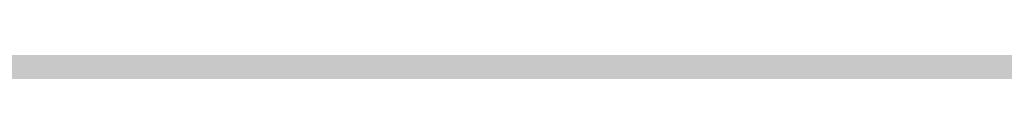
# Model space of a CAD drawing. Units: feet. Extents: x 3168 to 4724, y 827 to 1477.
# Tile 239 of 256: x 3382.8822 to 3383.8327, y 1099.0007 to 1099.0148. Entities that reach past the tile are written whole.
import ezdxf

# ---------------------------------------------------------------- set-up
doc = ezdxf.new("R2010")
doc.units = ezdxf.units.FT
doc.layers.add('A-ELEV', color=7, linetype='Continuous', lineweight=35)
doc.layers.add('A-ELEV-PATT', color=8, linetype='Continuous', lineweight=13)

msp = doc.modelspace()

# ---------------------------------------------------------------- hatches: boundary and pattern name
at = {"layer": 'A-ELEV-PATT'}
h = msp.add_hatch(color=256, dxfattribs=at)
h.dxf.hatch_style = 1
edge = h.paths.add_edge_path()
edge.add_ellipse((3552.90576, 979.22014), major_axis=(36.74492, 0), ratio=0.48484848, start_angle=0, end_angle=360)
edge = h.paths.add_edge_path()
edge.add_ellipse((3559.89164, 929.25228), major_axis=(36.74492, 0), ratio=0.48484848, start_angle=0, end_angle=360)
edge = h.paths.add_edge_path()
edge.add_line((3299.31681, 1198.60608), (3479.91671, 1198.60608))
edge.add_line((3479.91671, 1198.60608), (3479.91671, 1209.86857))
edge.add_spline(control_points=[(3479.91671, 1209.86857), (3464.30116, 1209.86857), (3448.6856, 1209.86857), (3410.94914, 1209.86857), (3388.82823, 1209.86857), (3355.64688, 1209.86857), (3344.58642, 1209.86857), (3327.99574, 1209.86857), (3322.46552, 1209.86857), (3314.17018, 1209.86857), (3311.40507, 1209.86857), (3307.2574, 1209.86857), (3305.87484, 1209.86857), (3303.801, 1209.86857), (3303.10973, 1209.86857), (3302.07281, 1209.86857), (3301.72717, 1209.86857), (3301.20871, 1209.86857), (3301.03589, 1209.86857), (3300.77666, 1209.86857), (3300.69025, 1209.86857), (3300.56064, 1209.86857), (3300.51743, 1209.86857), (3300.45263, 1209.86857), (3300.43102, 1209.86857), (3300.39862, 1209.86857), (3300.38782, 1209.86857), (3300.36622, 1209.86857), (3300.34568, 1209.86857), (3300.34555, 1209.86857), (3300.3455, 1209.86857), (3300.3433, 1209.86857), (3300.34115, 1209.86857), (3300.33791, 1209.86857), (3300.33683, 1209.86857), (3300.33394, 1209.86857), (3300.33213, 1209.86857), (3300.32552, 1209.86858), (3300.32071, 1209.86858), (3300.31092, 1209.86859), (3300.30595, 1209.8686), (3300.29051, 1209.86862), (3300.28005, 1209.86865), (3300.23243, 1209.86878), (3300.1953, 1209.86895), (3299.95107, 1209.87061), (3299.74482, 1209.87433), (3299.43683, 1209.88326), (3299.33439, 1209.88679), (3299.18108, 1209.89292), (3299.13003, 1209.8951), (3298.65222, 1209.9168), (3298.22946, 1209.94572), (3297.60163, 1210.00237), (3297.3934, 1210.02346), (3297.08265, 1210.05831), (3296.97933, 1210.07046), (3296.29295, 1210.15486), (3295.71815, 1210.24336), (3294.86872, 1210.39885), (3294.5877, 1210.45448), (3294.16934, 1210.54335), (3294.03042, 1210.57388), (3291.70715, 1211.1012), (3289.65359, 1211.81344), (3285.77626, 1213.56399), (3283.95141, 1214.60348), (3280.51216, 1216.98008), (3278.89724, 1218.31759), (3276.37991, 1220.82949), (3275.41604, 1221.91774), (3274.03934, 1223.7077), (3273.58104, 1224.34953), (3273.14323, 1225.01632)], knot_values=[39.119033, 39.119033, 39.119033, 39.119033, 39.286353, 39.286353, 39.523379, 39.523379, 39.641892, 39.641892, 39.701148, 39.701148, 39.730777, 39.730777, 39.745591, 39.745591, 39.752998, 39.752998, 39.756701, 39.756701, 39.758553, 39.758553, 39.759479, 39.759479, 39.759942, 39.759942, 39.760173, 39.760173, 39.760289, 39.760289, 39.760405, 39.760405, 39.760463, 39.760463, 39.763389, 39.763389, 39.764851, 39.764851, 39.767304, 39.767304, 39.773825, 39.773825, 39.78057, 39.78057, 39.79477, 39.79477, 39.845194, 39.845194, 40.126715, 40.126715, 40.267476, 40.267476, 40.337856, 40.337856, 40.927023, 40.927023, 41.221606, 41.221606, 41.368898, 41.368898, 42.202622, 42.202622, 42.619485, 42.619485, 42.827916, 42.827916, 46.118323, 46.118323, 49.408731, 49.408731, 52.699139, 52.699139, 54.927489, 54.927489, 56.104228, 56.104228, 56.104228, 56.104228], weights=[1, 1, 1, 1, 1, 1, 1, 1, 1, 1, 1, 1, 1, 1, 1, 1, 1, 1, 1, 1, 1, 1, 1, 1, 1, 1, 1, 1, 1, 1, 1, 1, 1, 1, 1, 1, 1, 1, 1, 1, 1, 1, 1, 1, 1, 1, 1, 1, 1, 1, 1, 1, 1, 1, 1, 1, 1, 1, 1, 1, 1, 1, 1, 1, 1, 1, 1, 1, 1, 1, 1, 1, 1, 1], degree=3, periodic=0)
edge.add_line((3273.14323, 1225.01632), (3273.14323, 1099.01632))
edge.add_line((3273.14323, 1099.01632), (3299.31681, 1099.01632))
edge.add_line((3299.31681, 1099.01632), (3299.31681, 1198.60608))
edge = h.paths.add_edge_path()
edge.add_line((3304.75844, 1324.15806), (3479.91671, 1324.15806))
edge.add_line((3479.91671, 1324.15806), (3479.91671, 1335.71462))
edge.add_line((3479.91671, 1335.71462), (3269.16163, 1335.71462))
edge.add_spline(control_points=[(3269.16163, 1335.71462), (3264.02423, 1335.71462), (3258.36412, 1328.95819), (3259.26431, 1323.90027)], knot_values=[0, 0, 0, 0, 15.412191, 15.412191, 15.412191, 15.412191], degree=3, periodic=0)
edge.add_line((3259.26431, 1323.90027), (3265.51685, 1288.76913))
edge.add_line((3265.51685, 1288.76913), (3275.2651, 1261.54563))
edge.add_line((3275.2651, 1261.54563), (3304.75844, 1261.54563))
edge.add_line((3304.75844, 1261.54563), (3304.75844, 1324.15806))
h = msp.add_hatch(color=256, dxfattribs=at)
h.dxf.hatch_style = 1
h.paths.add_polyline_path([(3384.52525, 1099.01632), (3335.02917, 1099.01632), (3299.31681, 1099.01632), (3273.14323, 1099.01632), (3217.56536, 1099.01632), (3168.06928, 827.11626), (3335.02917, 827.11626)])

# ---------------------------------------------------------------- linework, layer by layer
at = {"layer": 'A-ELEV'}
msp.add_open_spline([(3808.5202, 1099.01632), (3808.5202, 1141.41324), (3808.5202, 1183.81015), (3808.5202, 1226.63532), (3808.5202, 1227.06358), (3808.5202, 1227.49183), (3811.49187, 1248.99467), (3814.46354, 1270.49752), (3817.46523, 1292.21756), (3817.49525, 1292.43476), (3817.52526, 1292.65196), (3817.5728, 1310.10675), (3817.62034, 1327.56153), (3817.66788, 1345.01632), (3817.66788, 1345.45796), (3817.66788, 1345.89961), (3817.66788, 1346.45605), (3817.66788, 1346.57084), (3817.66788, 1346.75289), (3817.66788, 1346.82014), (3817.66788, 1346.93487), (3817.66788, 1346.98234), (3817.66788, 1347.03859), (3817.66788, 1347.04736), (3817.66788, 1347.07366), (3817.66788, 1347.0593), (3817.66788, 1347.06155), (3817.66788, 1347.06267), (3817.66788, 1347.06603), (3817.66787, 1347.06827), (3817.66787, 1347.075), (3817.66787, 1347.07949), (3817.66785, 1347.09294), (3817.66783, 1347.1019), (3817.66777, 1347.12879), (3817.6677, 1347.1467), (3817.66743, 1347.20042), (3817.66716, 1347.23619), (3817.6661, 1347.34338), (3817.66504, 1347.41469), (3817.66081, 1347.62809), (3817.65661, 1347.76971), (3817.63997, 1348.19249), (3817.62351, 1348.47159), (3817.55909, 1349.30007), (3817.49612, 1349.84059), (3817.25543, 1351.42416), (3817.02632, 1352.42879), (3816.30687, 1354.88891), (3815.74375, 1356.26873), (3814.46396, 1358.81921), (3813.74641, 1359.99097), (3812.19584, 1362.17234), (3811.36225, 1363.18212), (3809.58884, 1365.06901), (3808.64882, 1365.94611), (3806.65426, 1367.57962), (3805.5997, 1368.33615), (3803.35289, 1369.72233), (3802.16054, 1370.35239), (3799.60081, 1371.45359), (3798.23269, 1371.92548), (3795.28008, 1372.63462), (3793.69315, 1372.87207), (3791.86944, 1372.92648), (3791.74086, 1372.92922), (3791.35337, 1372.9341), (3791.09271, 1372.9329), (3790.30412, 1372.91507), (3789.76954, 1372.88419), (3789.20919, 1372.83024), (3789.19062, 1372.82842), (3789.13489, 1372.82291), (3789.0977, 1372.81914), (3789.04844, 1372.81401), (3789.0364, 1372.81274), (3789.00026, 1372.80892), (3788.97615, 1372.80633), (3788.9494, 1372.8034), (3788.94679, 1372.80312), (3788.94257, 1372.80266), (3788.94097, 1372.80248), (3788.93857, 1372.80222), (3788.93778, 1372.80213), (3788.93539, 1372.80187), (3788.86753, 1372.7944), (3788.75687, 1372.78223), (3788.70153, 1372.77614), (3788.53553, 1372.75788), (3788.42486, 1372.74571), (3788.09286, 1372.70918), (3787.87152, 1372.68484), (3787.20751, 1372.61179), (3786.76483, 1372.5631), (3785.43681, 1372.41701), (3784.55147, 1372.31962), (3781.89542, 1372.02744), (3780.12473, 1371.83266), (3774.81265, 1371.24831), (3771.27126, 1370.85874), (3760.64709, 1369.69004), (3753.56431, 1368.9109), (3732.31597, 1366.5735), (3718.15042, 1365.01523), (3694.00676, 1362.35933), (3684.02866, 1361.26169), (3674.05056, 1360.16406), (3664.60066, 1360.16406), (3655.15077, 1360.16406), (3626.80108, 1360.16406), (3607.90129, 1360.16406), (3551.20192, 1360.16406), (3513.40234, 1360.16406), (3467.72518, 1360.16406), (3459.8476, 1360.16406), (3436.21487, 1360.16406), (3420.45972, 1360.16406), (3373.19425, 1360.16406), (3341.68395, 1360.16406), (3302.84816, 1360.16406), (3295.52269, 1360.16406), (3286.03829, 1360.16406), (3283.87937, 1360.16406), (3277.40261, 1360.16406), (3273.08477, 1360.16406), (3267.73285, 1360.16406), (3266.69877, 1360.16406), (3263.59652, 1360.16406), (3261.52835, 1360.16406), (3259.23694, 1360.16406), (3259.0137, 1360.16406), (3258.34396, 1360.16406), (3257.89747, 1360.16406), (3257.431, 1360.16406), (3257.41102, 1360.16406), (3257.37057, 1360.16406), (3257.37547, 1360.16406), (3257.3746, 1360.16406), (3257.37394, 1360.16406), (3257.37196, 1360.16406), (3257.37064, 1360.16406), (3257.36667, 1360.16406), (3257.36403, 1360.16406), (3257.35611, 1360.16405), (3257.35083, 1360.16405), (3257.33499, 1360.16402), (3257.32443, 1360.164), (3257.29277, 1360.1639), (3257.27168, 1360.1638), (3257.20844, 1360.1634), (3257.16634, 1360.163), (3257.04021, 1360.16139), (3256.95635, 1360.15978), (3256.7055, 1360.15339), (3256.53924, 1360.14704), (3256.04357, 1360.12192), (3255.7173, 1360.0971), (3254.75245, 1360.00048), (3254.12797, 1359.90651), (3252.18007, 1359.52533), (3250.94157, 1359.14399), (3248.67018, 1358.24329), (3247.63574, 1357.72383), (3245.73263, 1356.60347), (3244.86339, 1356.00206), (3243.25311, 1354.74287), (3242.51197, 1354.08473), (3240.75105, 1352.34478), (3239.80096, 1351.22957), (3238.08777, 1348.87244), (3237.32469, 1347.63036), (3235.98251, 1344.97163), (3235.40221, 1343.55491), (3234.59108, 1340.81546), (3234.31088, 1339.54355), (3233.97649, 1336.80256), (3233.92211, 1335.33088), (3234.14892, 1332.59127), (3234.34953, 1331.3672), (3234.71989, 1329.99937), (3234.75242, 1329.88336), (3234.85362, 1329.5348), (3234.92589, 1329.30168), (3235.02484, 1329.00255), (3235.04692, 1328.93693), (3235.07764, 1328.84724), (3235.08592, 1328.8232), (3235.11094, 1328.75106), (3235.12783, 1328.70296), (3235.14799, 1328.64624), (3235.15106, 1328.63763), (3235.1561, 1328.62353), (3235.15806, 1328.61803), (3235.16021, 1328.61203), (3235.16561, 1328.59694), (3235.1801, 1328.55649), (3235.19026, 1328.5281), (3235.22076, 1328.44295), (3235.24108, 1328.38618), (3235.30207, 1328.21587), (3235.34273, 1328.10232), (3235.4647, 1327.7617), (3235.54601, 1327.53462), (3235.78995, 1326.85338), (3235.95258, 1326.39922), (3236.44046, 1325.03674), (3236.76571, 1324.12841), (3237.74148, 1321.40345), (3238.39198, 1319.5868), (3240.34351, 1314.13687), (3241.64452, 1310.50358), (3245.54757, 1299.60371), (3248.14961, 1292.33713), (3255.95571, 1270.53739), (3261.15977, 1256.00423), (3267.38762, 1238.612), (3268.4114, 1235.75294), (3269.51038, 1232.68386), (3269.58558, 1232.47385), (3269.70661, 1232.13585), (3269.75244, 1232.00786), (3269.82733, 1231.79873), (3269.85638, 1231.7176), (3269.90632, 1231.57812), (3269.92721, 1231.51978), (3269.97247, 1231.39341), (3269.99683, 1231.32537), (3270.0265, 1231.24251), (3270.03181, 1231.22768), (3270.04028, 1231.20402), (3270.03922, 1231.20698), (3270.03936, 1231.2066), (3270.03943, 1231.20641), (3270.03963, 1231.20585), (3270.03977, 1231.20547), (3270.04017, 1231.20433), (3270.04044, 1231.20358), (3270.04125, 1231.20131), (3270.0418, 1231.1998), (3270.04342, 1231.19527), (3270.0445, 1231.19225), (3270.04776, 1231.18318), (3270.04993, 1231.17714), (3270.05644, 1231.15903), (3270.06079, 1231.14696), (3270.07387, 1231.11076), (3270.08261, 1231.08666), (3270.10894, 1231.01441), (3270.1266, 1230.96635), (3270.17993, 1230.82246), (3270.21595, 1230.72692), (3270.32532, 1230.44151), (3270.40003, 1230.25281), (3270.62925, 1229.69144), (3270.78888, 1229.3235), (3271.28649, 1228.23832), (3271.6431, 1227.53975), (3272.77586, 1225.51528), (3273.61417, 1224.2605), (3275.41604, 1221.91774), (3276.37991, 1220.82949), (3278.89724, 1218.31759), (3280.51216, 1216.98008), (3283.95141, 1214.60348), (3285.77626, 1213.56399), (3289.65359, 1211.81344), (3291.70715, 1211.1012), (3294.03042, 1210.57388), (3294.16934, 1210.54335), (3294.5877, 1210.45448), (3294.86872, 1210.39885), (3295.71815, 1210.24336), (3296.29295, 1210.15486), (3296.97933, 1210.07046), (3297.08265, 1210.05831), (3297.3934, 1210.02346), (3297.60163, 1210.00237), (3298.22946, 1209.94572), (3298.65222, 1209.9168), (3299.13003, 1209.8951), (3299.18108, 1209.89292), (3299.33439, 1209.88679), (3299.43683, 1209.88326), (3299.74482, 1209.87433), (3299.95107, 1209.87061), (3300.1953, 1209.86895), (3300.23243, 1209.86878), (3300.28005, 1209.86865), (3300.29051, 1209.86862), (3300.30595, 1209.8686), (3300.31092, 1209.86859), (3300.32071, 1209.86858), (3300.32552, 1209.86858), (3300.33213, 1209.86857), (3300.33394, 1209.86857), (3300.33683, 1209.86857), (3300.33791, 1209.86857), (3300.34115, 1209.86857), (3300.3433, 1209.86857), (3300.3455, 1209.86857), (3300.34555, 1209.86857), (3300.34568, 1209.86857), (3300.36622, 1209.86857), (3300.38782, 1209.86857), (3300.39862, 1209.86857), (3300.43102, 1209.86857), (3300.45263, 1209.86857), (3300.51743, 1209.86857), (3300.56064, 1209.86857), (3300.69025, 1209.86857), (3300.77666, 1209.86857), (3301.03589, 1209.86857), (3301.20871, 1209.86857), (3301.72717, 1209.86857), (3302.07281, 1209.86857), (3303.10973, 1209.86857), (3303.801, 1209.86857), (3305.87484, 1209.86857), (3307.2574, 1209.86857), (3311.40507, 1209.86857), (3314.17018, 1209.86857), (3322.46552, 1209.86857), (3327.99574, 1209.86857), (3344.58642, 1209.86857), (3355.64688, 1209.86857), (3388.82823, 1209.86857), (3410.94914, 1209.86857), (3477.31185, 1209.86857), (3521.55366, 1209.86857), (3566.83618, 1209.86857), (3567.87689, 1209.86857), (3570.99902, 1209.86857), (3573.08043, 1209.86857), (3575.7814, 1209.86857), (3576.40094, 1209.86857), (3577.29582, 1209.86857), (3577.57115, 1209.86857), (3578.39715, 1209.86857), (3578.94781, 1209.86857), (3579.75649, 1209.86857), (3580.01451, 1209.86857), (3580.34274, 1209.86857), (3580.32686, 1209.86857), (3580.32717, 1209.86857), (3580.32732, 1209.86857), (3580.32778, 1209.86857), (3580.32809, 1209.86857), (3580.329, 1209.86857), (3580.32961, 1209.86857), (3580.33145, 1209.86857), (3580.33267, 1209.86857), (3580.33633, 1209.86857), (3580.33878, 1209.86857), (3580.34611, 1209.86856), (3580.35099, 1209.86856), (3580.36566, 1209.86854), (3580.37544, 1209.86852), (3580.4048, 1209.86845), (3580.42439, 1209.86838), (3580.48318, 1209.86808), (3580.52244, 1209.86779), (3580.64036, 1209.86662), (3580.71919, 1209.86545), (3580.95632, 1209.86077), (3581.11522, 1209.85607), (3581.59416, 1209.83723), (3581.91642, 1209.81833), (3582.88995, 1209.74243), (3583.54799, 1209.66617), (3585.53183, 1209.36062), (3586.86722, 1209.05389), (3589.47155, 1208.25247), (3590.74024, 1207.75785), (3591.99545, 1207.1588), (3592.05781, 1207.12874), (3592.24424, 1207.03795), (3592.36768, 1206.97663), (3592.73528, 1206.79036), (3592.97675, 1206.6631), (3593.24454, 1206.51644), (3593.27473, 1206.49982), (3593.36512, 1206.44984), (3593.42511, 1206.41633), (3593.60431, 1206.31529), (3593.72273, 1206.24721), (3593.85721, 1206.1684), (3593.87436, 1206.15832), (3593.92574, 1206.12804), (3593.9599, 1206.1078), (3594.06209, 1206.0469), (3594.12983, 1206.00607), (3594.20844, 1205.95817), (3594.21968, 1205.9513), (3594.25339, 1205.93069), (3594.27582, 1205.91692), (3594.34297, 1205.87554), (3594.38756, 1205.84785), (3594.43362, 1205.81905), (3594.43526, 1205.81802), (3594.44017, 1205.81495), (3594.44345, 1205.81289), (3594.44712, 1205.81059), (3594.44752, 1205.81035), (3594.44869, 1205.80961), (3594.44948, 1205.80912), (3594.45037, 1205.80856), (3594.45047, 1205.8085), (3594.4506, 1205.80842), (3594.4674, 1205.79789), (3594.49327, 1205.78167), (3594.5062, 1205.77357), (3594.54501, 1205.74925), (3594.57088, 1205.73303), (3594.64849, 1205.6844), (3594.70023, 1205.65197), (3594.85544, 1205.55469), (3594.95892, 1205.48984), (3595.26936, 1205.29528), (3595.47631, 1205.16558), (3596.09719, 1204.77646), (3596.5111, 1204.51705), (3597.75284, 1203.73883), (3598.58067, 1203.22001), (3601.06415, 1201.66355), (3602.71981, 1200.62591), (3607.68677, 1197.513), (3610.99809, 1195.43773), (3620.93202, 1189.2119), (3627.55464, 1185.06135), (3647.42251, 1172.60971), (3660.66775, 1164.30861), (3700.40348, 1139.40531), (3726.89397, 1122.80312), (3757.20572, 1103.80605), (3761.02697, 1101.41118), (3764.84822, 1099.01632), (3745.32827, 1099.01632), (3725.80832, 1099.01632), (3706.28837, 1099.01632), (3706.28837, 1108.45324), (3706.28837, 1117.89016), (3706.28837, 1127.32708), (3710.75075, 1127.32708), (3715.21314, 1127.32708), (3719.67553, 1127.32708)], degree=3, knots=[0, 0, 0, 0, 0.982037, 0.982037, 0.991957, 0.991957, 0.991957, 1.966522, 1.966522, 1.976367, 1.976367, 1.976367, 2.976367, 2.976367, 2.976367, 3.00169, 3.00169, 3.008272, 3.008272, 3.012129, 3.012129, 3.014851, 3.014851, 3.015353, 3.015353, 3.016359, 3.016359, 3.017365, 3.017365, 3.019376, 3.019376, 3.023398, 3.023398, 3.031442, 3.031442, 3.047531, 3.047531, 3.079708, 3.079708, 3.144063, 3.144063, 3.272772, 3.272772, 3.53019, 3.53019, 4.045026, 4.045026, 5.074698, 5.074698, 6.700878, 6.700878, 8.327058, 8.327058, 9.953238, 9.953238, 11.579418, 11.579418, 13.205598, 13.205598, 14.831778, 14.831778, 16.457958, 16.457958, 18.084138, 18.084138, 18.206872, 18.206872, 18.45234, 18.45234, 18.943275, 18.943275, 18.960093, 18.960093, 18.993729, 18.993729, 19.00461, 19.00461, 19.026374, 19.026374, 19.028737, 19.028737, 19.03018, 19.03018, 19.030897, 19.030897, 19.032332, 19.032332, 19.033766, 19.033766, 19.036636, 19.036636, 19.042374, 19.042374, 19.053851, 19.053851, 19.076805, 19.076805, 19.122714, 19.122714, 19.21453, 19.21453, 19.398163, 19.398163, 19.765429, 19.765429, 20.024128, 20.024128, 20.024128, 20.092031, 20.092031, 20.227836, 20.227836, 20.499446, 20.499446, 20.556051, 20.556051, 20.66926, 20.66926, 20.895678, 20.895678, 20.948316, 20.948316, 20.963829, 20.963829, 20.994855, 20.994855, 21.002285, 21.002285, 21.017146, 21.017146, 21.01875, 21.01875, 21.021959, 21.021959, 21.022102, 21.022102, 21.022249, 21.022249, 21.022708, 21.022708, 21.023627, 21.023627, 21.025464, 21.025464, 21.029138, 21.029138, 21.036486, 21.036486, 21.051183, 21.051183, 21.080575, 21.080575, 21.139361, 21.139361, 21.256932, 21.256932, 21.492073, 21.492073, 21.962356, 21.962356, 23.01002, 23.01002, 24.057684, 24.057684, 25.105348, 25.105348, 26.153011, 26.153011, 27.776787, 27.776787, 29.400562, 29.400562, 31.024337, 31.024337, 32.278801, 32.278801, 33.533265, 33.533265, 34.467568, 34.467568, 34.553971, 34.553971, 34.726776, 34.726776, 34.775309, 34.775309, 34.793079, 34.793079, 34.82862, 34.82862, 34.834979, 34.834979, 34.839039, 34.839039, 34.839411, 34.839411, 34.840285, 34.840285, 34.842034, 34.842034, 34.845531, 34.845531, 34.852525, 34.852525, 34.866512, 34.866512, 34.894488, 34.894488, 34.950439, 34.950439, 35.062342, 35.062342, 35.286147, 35.286147, 35.733758, 35.733758, 35.821815, 35.821815, 35.828283, 35.828283, 35.832225, 35.832225, 35.834724, 35.834724, 35.836521, 35.836521, 35.838617, 35.838617, 35.839073, 35.839073, 35.839345, 35.839345, 35.839617, 35.839617, 35.840161, 35.840161, 35.841249, 35.841249, 35.843425, 35.843425, 35.847778, 35.847778, 35.856482, 35.856482, 35.873891, 35.873891, 35.908709, 35.908709, 35.978345, 35.978345, 36.117617, 36.117617, 36.396161, 36.396161, 36.953248, 36.953248, 38.067423, 38.067423, 40.295772, 40.295772, 42.524122, 42.524122, 45.81453, 45.81453, 49.104937, 49.104937, 52.395345, 52.395345, 52.603776, 52.603776, 53.020639, 53.020639, 53.854363, 53.854363, 54.001655, 54.001655, 54.296238, 54.296238, 54.885405, 54.885405, 54.955785, 54.955785, 55.096546, 55.096546, 55.378067, 55.378067, 55.42849, 55.42849, 55.442691, 55.442691, 55.449436, 55.449436, 55.455957, 55.455957, 55.458409, 55.458409, 55.459872, 55.459872, 55.462798, 55.462798, 55.462856, 55.462856, 55.462972, 55.462972, 55.463088, 55.463088, 55.463319, 55.463319, 55.463782, 55.463782, 55.464708, 55.464708, 55.46656, 55.46656, 55.470263, 55.470263, 55.47767, 55.47767, 55.492484, 55.492484, 55.522112, 55.522112, 55.581369, 55.581369, 55.699882, 55.699882, 55.936907, 55.936907, 56.410959, 56.410959, 56.42211, 56.42211, 56.444413, 56.444413, 56.451051, 56.451051, 56.454001, 56.454001, 56.459901, 56.459901, 56.462666, 56.462666, 56.463418, 56.463418, 56.464171, 56.464171, 56.465675, 56.465675, 56.468684, 56.468684, 56.474702, 56.474702, 56.486738, 56.486738, 56.51081, 56.51081, 56.558955, 56.558955, 56.655243, 56.655243, 56.847821, 56.847821, 57.232975, 57.232975, 58.003284, 58.003284, 59.543901, 59.543901, 62.625137, 62.625137, 68.787607, 68.787607, 74.950078, 74.950078, 75.27336, 75.27336, 75.919923, 75.919923, 77.213051, 77.213051, 77.377769, 77.377769, 77.707206, 77.707206, 78.366079, 78.366079, 78.462532, 78.462532, 78.655436, 78.655436, 79.041245, 79.041245, 79.105735, 79.105735, 79.234714, 79.234714, 79.492672, 79.492672, 79.502197, 79.502197, 79.521249, 79.521249, 79.523534, 79.523534, 79.528103, 79.528103, 79.528682, 79.528682, 79.528885, 79.528885, 79.529089, 79.529089, 79.529495, 79.529495, 79.530308, 79.530308, 79.531935, 79.531935, 79.535187, 79.535187, 79.541693, 79.541693, 79.554704, 79.554704, 79.580725, 79.580725, 79.632769, 79.632769, 79.736856, 79.736856, 79.94503, 79.94503, 80.361377, 80.361377, 80.421435, 80.421435, 80.421435, 81.421435, 81.421435, 81.421435, 82.421435, 82.421435, 82.421435, 83.421435, 83.421435, 83.421435, 83.421435], dxfattribs=at)

doc.saveas('drawing.dxf')
